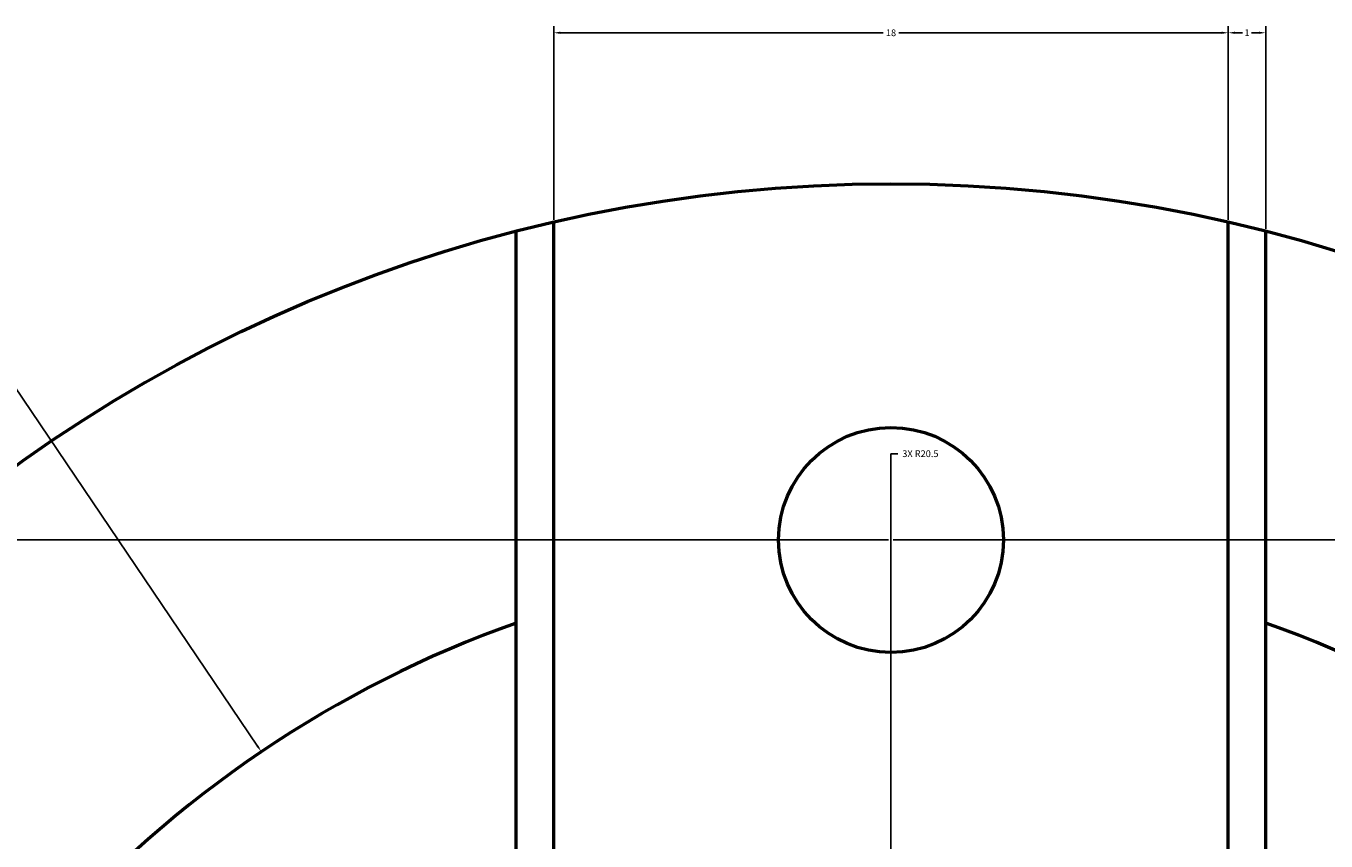
# Model space of a CAD drawing. Units: inches. Extents: x -19.9 to 72.3, y -39.8 to 57.5.
# Tile 7 of 8: x 5 to 39.7, y 35.8 to 57.5. Entities that reach past the tile are written whole.
import ezdxf

# ---------------------------------------------------------------- set-up
doc = ezdxf.new("R2010")
doc.units = ezdxf.units.IN
doc.header["$MEASUREMENT"] = 0
for name, color, linetype, lineweight in [('M-DIMS', 2, 'Continuous', 18), ('M-OUTL', 7, 'Continuous', 50), ('M-OUTL-HOLE', 7, 'Continuous', 50), ('M-OUTL-SLOT', 7, 'Continuous', 50)]:
    doc.layers.add(name, color=color, linetype=linetype, lineweight=lineweight)
doc.styles.get("Standard").update_dxf_attribs({"font": 'arial.ttf'})
doc.dimstyles.get("Standard").update_dxf_attribs({"dimtxt": 0.18, "dimasz": 0.18, "dimexe": 0.18, "dimexo": 0.0625, "dimgap": 0.09, "dimtad": 0, "dimtih": 1, "dimtoh": 1, "dimdec": 4, "dimzin": 0, "dimdsep": 46, "dimtxsty": 'Standard', "dimcen": 0.09, "dimadec": 0, "dimazin": 0, "dimtfac": 1, "dimtdec": 4, "dimtofl": 0, "dimtmove": 0, "dimatfit": 3, "dimfxl": 1, "dimtolj": 1, "dimtzin": 0, "dimarcsym": 0})

# ---------------------------------------------------------------- blocks, each defined once
blk = doc.blocks.new('FLANGE-MOUNT-D8-RELIEVED')
for start, end in [(109.4712, 138.6562), (161.3438, 190.5288)]:
    blk.add_arc((26.414, -15.25), 30, start, end)
blk = doc.blocks.new('FLANGE-HOLE-D6')
blk.add_circle((0, 0), 3)
blk = doc.blocks.new('FLANGE-STRAIGHT-SLOT')
for p, q in [((0, 0), (0, 21.114)), ((1, -0.54), (1, 20.869))]:
    blk.add_line(p, q)
blk = doc.blocks.new('*D6')
at = {"layer": 'Defpoints', "color": 0, "transparency": 16777216}
for p in [(28.06, 43.841), (28.06, -17.159), (72.086, -17.159)]:
    blk.add_point(p, dxfattribs=at)
at = {"layer": 'M-DIMS', "color": 0, "lineweight": -2, "transparency": 16777216}
for p, q in [((28.122, 43.841), (72.266, 43.841)), ((72.086, 43.661), (72.086, 13.523)), ((72.086, -16.979), (72.086, 13.159)), ((28.122, -17.159), (72.266, -17.159))]:
    blk.add_line(p, q, dxfattribs=at)
at = {"layer": 'M-DIMS', "color": 0, "transparency": 16777216}
for points in [[(72.056, 43.661), (72.116, 43.661), (72.086, 43.841)], [(72.056, -16.979), (72.116, -16.979), (72.086, -17.159)]]:
    blk.add_solid(points, dxfattribs=at)
at = {"layer": 'M-DIMS', "color": 0, "transparency": 16777216, "insert": (72.086, 13.341), "char_height": 0.18, "attachment_point": 5}
blk.add_mtext('\\A1;61', dxfattribs=at)
blk = doc.blocks.new('*D7')
at = {"layer": 'Defpoints', "color": 0, "transparency": 16777216}
for p in [(37.06, 57.367), (19.06, 52.316), (37.06, 52.316)]:
    blk.add_point(p, dxfattribs=at)
at = {"layer": 'M-DIMS', "color": 0, "lineweight": -2, "transparency": 16777216}
for p, q in [((19.06, 52.378), (19.06, 57.547)), ((19.24, 57.367), (27.849, 57.367)), ((36.88, 57.367), (28.271, 57.367)), ((37.06, 52.378), (37.06, 57.547))]:
    blk.add_line(p, q, dxfattribs=at)
at = {"layer": 'M-DIMS', "color": 0, "transparency": 16777216}
for points in [[(19.24, 57.397), (19.24, 57.337), (19.06, 57.367)], [(36.88, 57.397), (36.88, 57.337), (37.06, 57.367)]]:
    blk.add_solid(points, dxfattribs=at)
at = {"layer": 'M-DIMS', "color": 0, "transparency": 16777216, "insert": (28.06, 57.367), "char_height": 0.18, "attachment_point": 5}
blk.add_mtext('\\A1;18', dxfattribs=at)
blk = doc.blocks.new('*D8')
at = {"layer": 'Defpoints', "color": 0, "transparency": 16777216}
for p in [(38.06, 57.367), (37.06, 52.316), (38.06, 52.071)]:
    blk.add_point(p, dxfattribs=at)
at = {"layer": 'M-DIMS', "color": 0, "lineweight": -2, "transparency": 16777216}
for p, q in [((37.06, 52.378), (37.06, 57.547)), ((37.24, 57.367), (37.437, 57.367)), ((37.88, 57.367), (37.683, 57.367)), ((38.06, 52.134), (38.06, 57.547))]:
    blk.add_line(p, q, dxfattribs=at)
at = {"layer": 'M-DIMS', "color": 0, "transparency": 16777216}
for points in [[(37.24, 57.397), (37.24, 57.337), (37.06, 57.367)], [(37.88, 57.397), (37.88, 57.337), (38.06, 57.367)]]:
    blk.add_solid(points, dxfattribs=at)
at = {"layer": 'M-DIMS', "color": 0, "transparency": 16777216, "insert": (37.56, 57.367), "char_height": 0.18, "attachment_point": 5}
blk.add_mtext('\\A1;1', dxfattribs=at)
blk = doc.blocks.new('*D10')
at = {"layer": 'Defpoints', "color": 0, "transparency": 16777216}
for p in [(28.06, 43.841), (-15.966, 28.591), (1.646, 28.591)]:
    blk.add_point(p, dxfattribs=at)
at = {"layer": 'M-DIMS', "color": 0, "lineweight": -2, "transparency": 16777216}
for p, q in [((27.997, 43.841), (-16.146, 43.841)), ((-15.966, 43.661), (-15.966, 36.398)), ((-15.966, 28.771), (-15.966, 36.034)), ((1.584, 28.591), (-16.146, 28.591))]:
    blk.add_line(p, q, dxfattribs=at)
at = {"layer": 'M-DIMS', "color": 0, "transparency": 16777216}
for points in [[(-15.996, 43.661), (-15.936, 43.661), (-15.966, 43.841)], [(-15.996, 28.771), (-15.936, 28.771), (-15.966, 28.591)]]:
    blk.add_solid(points, dxfattribs=at)
at = {"layer": 'M-DIMS', "color": 0, "transparency": 16777216, "insert": (-15.966, 36.216), "char_height": 0.18, "attachment_point": 5}
blk.add_mtext('\\A1;15.25', dxfattribs=at)
blk = doc.blocks.new('*D11')
at = {"layer": 'Defpoints', "color": 0, "transparency": 16777216}
for p in [(5.703, 46.51), (50.417, -19.828)]:
    blk.add_point(p, dxfattribs=at)
at = {"layer": 'M-DIMS', "color": 0, "lineweight": -2, "transparency": 16777216}
for p, q in [((27.97, 13.341), (28.15, 13.341)), ((28.06, 13.251), (28.06, 13.431)), ((63.831, -39.729), (50.517, -19.977)), ((64.011, -39.729), (63.831, -39.729))]:
    blk.add_line(p, q, dxfattribs=at)
at = {"layer": 'M-DIMS', "color": 0, "transparency": 16777216}
blk.add_solid([(50.542, -19.96), (50.492, -19.994), (50.417, -19.828)], dxfattribs=at)
at = {"layer": 'M-DIMS', "color": 0, "transparency": 16777216, "insert": (64.327, -39.729), "char_height": 0.18, "attachment_point": 5}
blk.add_mtext('\\A1;∅80', dxfattribs=at)
blk = doc.blocks.new('*D13')
at = {"layer": 'Defpoints', "color": 0, "transparency": 16777216}
for p in [(11.256, 38.194), (28.06, 13.341)]:
    blk.add_point(p, dxfattribs=at)
at = {"layer": 'M-DIMS', "color": 0, "lineweight": -2, "transparency": 16777216}
for p, q in [((0.994, 53.105), (1.174, 53.105)), ((1.174, 53.105), (11.155, 38.343)), ((27.97, 13.341), (28.15, 13.341)), ((28.06, 13.251), (28.06, 13.431))]:
    blk.add_line(p, q, dxfattribs=at)
at = {"layer": 'M-DIMS', "color": 0, "transparency": 16777216}
blk.add_solid([(11.18, 38.36), (11.131, 38.326), (11.256, 38.194)], dxfattribs=at)
at = {"layer": 'M-DIMS', "color": 0, "transparency": 16777216, "insert": (0.434, 53.105), "char_height": 0.18, "attachment_point": 5}
blk.add_mtext('\\A1;10X R30', dxfattribs=at)
blk = doc.blocks.new('*D14')
at = {"layer": 'Defpoints', "color": 0, "transparency": 16777216}
for p in [(28.06, 33.841), (28.06, 13.341)]:
    blk.add_point(p, dxfattribs=at)
at = {"layer": 'M-DIMS', "color": 0, "lineweight": -2, "transparency": 16777216}
for p, q in [((28.24, 46.141), (28.06, 46.141)), ((28.06, 46.141), (28.06, 34.021)), ((27.97, 13.341), (28.15, 13.341)), ((28.06, 13.251), (28.06, 13.431))]:
    blk.add_line(p, q, dxfattribs=at)
at = {"layer": 'M-DIMS', "color": 0, "transparency": 16777216}
blk.add_solid([(28.03, 34.021), (28.09, 34.021), (28.06, 33.841)], dxfattribs=at)
at = {"layer": 'M-DIMS', "color": 0, "transparency": 16777216, "insert": (28.844, 46.141), "char_height": 0.18, "attachment_point": 5}
blk.add_mtext('\\A1;3X R20.5', dxfattribs=at)

msp = doc.modelspace()

# ---------------------------------------------------------------- linework, layer by layer
at = {"layer": 'M-OUTL'}
msp.add_circle((28.06, 13.341), 40, dxfattribs=at)

# ---------------------------------------------------------------- block references
at = {"layer": 'M-OUTL-HOLE'}
for name, p in [('FLANGE-HOLE-D6', (28.06, 43.841)), ('FLANGE-MOUNT-D8-RELIEVED', (1.646, 28.591))]:
    msp.add_blockref(name, p, dxfattribs=at)
at = {"layer": 'M-OUTL-HOLE', "rotation": 240}
msp.add_blockref('FLANGE-MOUNT-D8-RELIEVED', (54.474, 28.591), dxfattribs=at)
at = {"layer": 'M-OUTL-SLOT', "extrusion": (0, 0, -1), "zscale": -1}
msp.add_blockref('FLANGE-STRAIGHT-SLOT', (-19.06, 31.202), dxfattribs=at)
at = {"layer": 'M-OUTL-SLOT'}
msp.add_blockref('FLANGE-STRAIGHT-SLOT', (37.06, 31.202), dxfattribs=at)

# ---------------------------------------------------------------- dimensions: what is measured, and where the dimension line sits
at = {"layer": 'M-DIMS'}
for base, p1, p2, picture, middle in [((37.06, 57.367), (19.06, 52.316), (37.06, 52.316), '*D7', (28.06, 57.367)), ((38.06, 57.367), (37.06, 52.316), (38.06, 52.071), '*D8', (37.56, 57.367))]:
    dim = msp.add_linear_dim(base=base, p1=p1, p2=p2, dimstyle='Standard', override={"dimdec": 0, "dimlfac": 1, "dimrnd": 0, "dimzin": 0, "dimdsep": 46, "dimlunit": 2}, dxfattribs=at)
    dim.commit()
    dim.dimension.update_dxf_attribs({"geometry": picture, "text_midpoint": middle})
for mpoint, text, override, picture, middle in [((11.256, 38.194), '10X <>', {"dimdec": 0, "dimlfac": 1, "dimrnd": 0, "dimzin": 0, "dimdsep": 46, "dimlunit": 2}, '*D13', (0.434, 53.105)), ((28.06, 33.841), '3X <>', {"dimdec": 1, "dimlfac": 1, "dimrnd": 0, "dimzin": 0, "dimdsep": 46, "dimlunit": 2}, '*D14', (28.844, 46.141))]:
    dim = msp.add_radius_dim(center=(28.06, 13.341), mpoint=mpoint, text=text, dimstyle='Standard', override=override, dxfattribs=at)
    dim.commit()
    dim.dimension.update_dxf_attribs({"geometry": picture, "text_midpoint": middle, "dimtype": 164})
dim = msp.add_diameter_dim_2p(p1=(5.703, 46.51), p2=(50.417, -19.828), dimstyle='Standard', override={"dimdec": 0, "dimlfac": 1, "dimrnd": 0, "dimzin": 0, "dimdsep": 46, "dimlunit": 2}, dxfattribs=at)
dim.commit()
dim.dimension.update_dxf_attribs({"geometry": '*D11', "text_midpoint": (64.327, -39.729), "dimtype": 163})
for base, p2, override, picture, middle in [((-15.966, 28.591), (1.646, 28.591), {"dimdec": 2, "dimlfac": 1, "dimrnd": 0, "dimzin": 0, "dimdsep": 46, "dimlunit": 2}, '*D10', (-15.966, 36.216)), ((72.086, -17.159), (28.06, -17.159), {"dimdec": 0, "dimlfac": 1, "dimrnd": 0, "dimzin": 0, "dimdsep": 46, "dimlunit": 2}, '*D6', (72.086, 13.341))]:
    dim = msp.add_linear_dim(base=base, p1=(28.06, 43.841), p2=p2, angle=90, dimstyle='Standard', override=override, dxfattribs=at)
    dim.commit()
    dim.dimension.update_dxf_attribs({"geometry": picture, "text_midpoint": middle})

doc.saveas('drawing.dxf')
